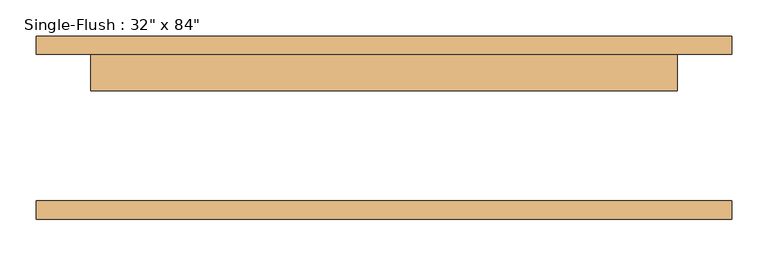
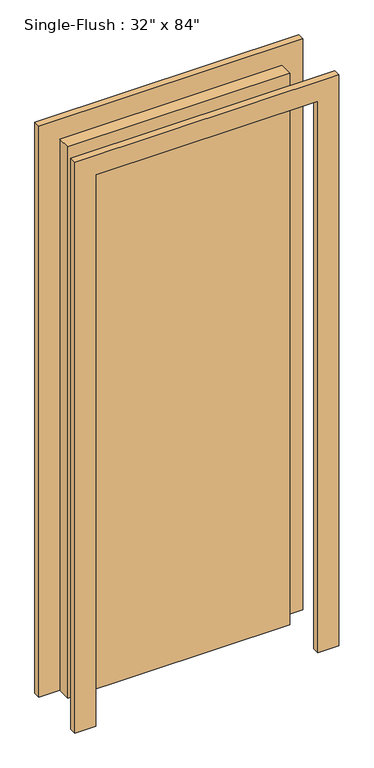
"""IFC4 building model written with IfcOpenShell, lengths in millimetres: door geometry."""

from ifc_helpers import new_model, si_unit, frame, origin, origin_with_axes, place, context, project, spatial, polyline, outline, extrude, source, transform, mapped, element, save


def door_64d5ae29(model_context):
    return source(origin(), model_context, "Body", "SweptSolid", [
        extrude(outline(polyline([(2209.8, -482.6), (0.0, -482.6), (0.0, -406.4), (2133.6, -406.4), (2133.6, 406.4), (0.0, 406.4), (0.0, 482.6), (2209.8, 482.6), (2209.8, -482.6)])), frame((0.0, 101.6, 0.0), z_axis=(0.0, 1.0, 0.0), x_axis=(0.0, 0.0, 1.0)), (0.0, 0.0, 1.0), 25.4),
        extrude(outline(polyline([(2209.8, 482.6), (2209.8, -482.6), (0.0, -482.6), (0.0, -406.4), (2133.6, -406.4), (2133.6, 406.4), (0.0, 406.4), (0.0, 482.6), (2209.8, 482.6)])), frame((0.0, -127.0, 0.0), z_axis=(0.0, 1.0, 0.0), x_axis=(0.0, 0.0, 1.0)), (0.0, 0.0, 1.0), 25.4),
        extrude(outline(polyline([(406.4, 50.8), (-406.4, 50.8), (-406.4, 101.6), (406.4, 101.6), (406.4, 50.8)])), origin_with_axes(), (0.0, 0.0, 1.0), 2133.6),
    ])


if __name__ == "__main__":
    model = new_model("IFC4")
    model_context = context("Model", 3, world=origin())
    ifc_project = project(units=[si_unit("LENGTHUNIT", "METRE", prefix="MILLI")], contexts=[model_context])
    site = spatial("IfcSite", under=ifc_project)
    building = spatial("IfcBuilding", under=site)
    placement = place(None, origin())
    door_shape = door_64d5ae29(model_context)
    element("IfcDoor", 1, ObjectType="Single-Flush : 32\" x 84\"", at=placement, inside=building, context=model_context, shape_type="MappedRepresentation", body=[
        mapped(door_shape, transform((0.0, 0.0, 0.0), x_axis=(1.0, 0.0, 0.0), y_axis=(0.0, 1.0, 0.0), z_axis=(0.0, 0.0, 1.0))),
    ])
    save(model, "model.ifc")

# Revit data of these elements
# Type "Single-Flush : 32\" x 84\""
#   Type Mark = "3"
#   Construction Type Id = "MDOOR"
#   Assembly Code = "C1020"
#   Analytic Construction = "Metal"
#   Thickness = 0' - 2"
#   Heat Transfer Coefficient (U) = 0.651978 BTU/(h·ft²·°F)
#   Height = 7' - 0"
#   Trim Projection Ext = 0' - 1"
#   Trim Projection Int = 0' - 1"
#   Trim Width = 0' - 3"
#   Width = 2' - 8"
#   Define Thermal Properties by = 1
#   Define Thermal Properties by = 1
#   Door Material = Door - Panel
#   Frame Material = Door - Frame
#   Visual Light Transmittance = 0
#   Solar Heat Gain Coefficient = 0
#   Function = (empty or 0)
#   Wall Closure = (empty or 0)
# Element 1 (IfcDoor, "Single-Flush : 32\" x 84\"")
#   Materials on its faces: "Door - Frame", "Door - Panel"
# Materials
#   "Door - Panel": class "Wood", colour RGB 210 159 95, transparency 0, Cost = 0
#   "Door - Frame": colour RGB 118 70 51, transparency 0, Cost = 0
